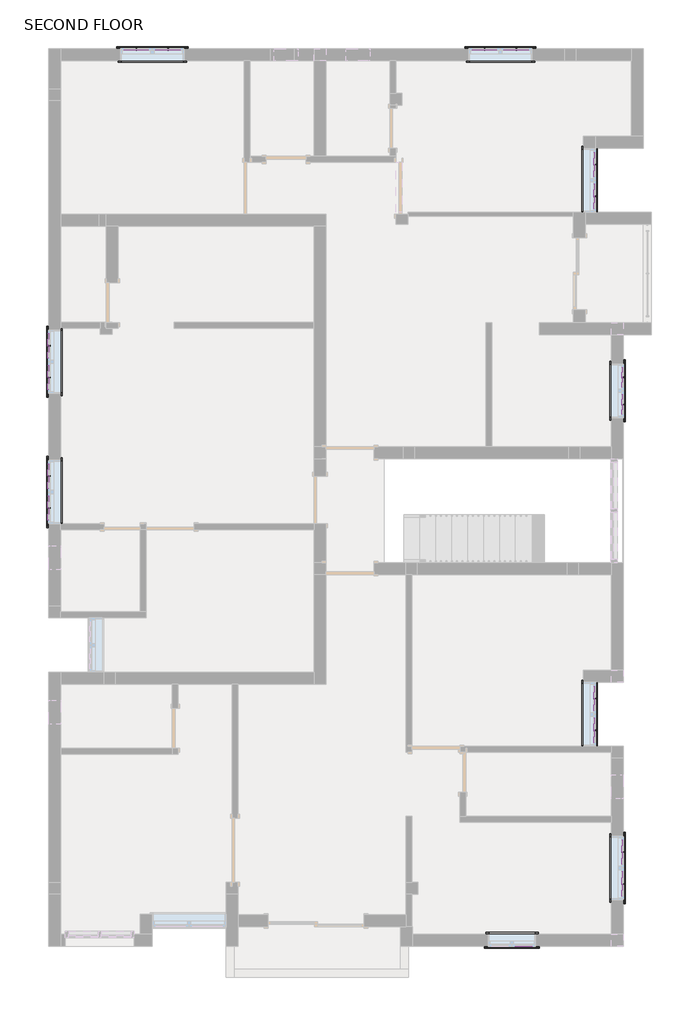
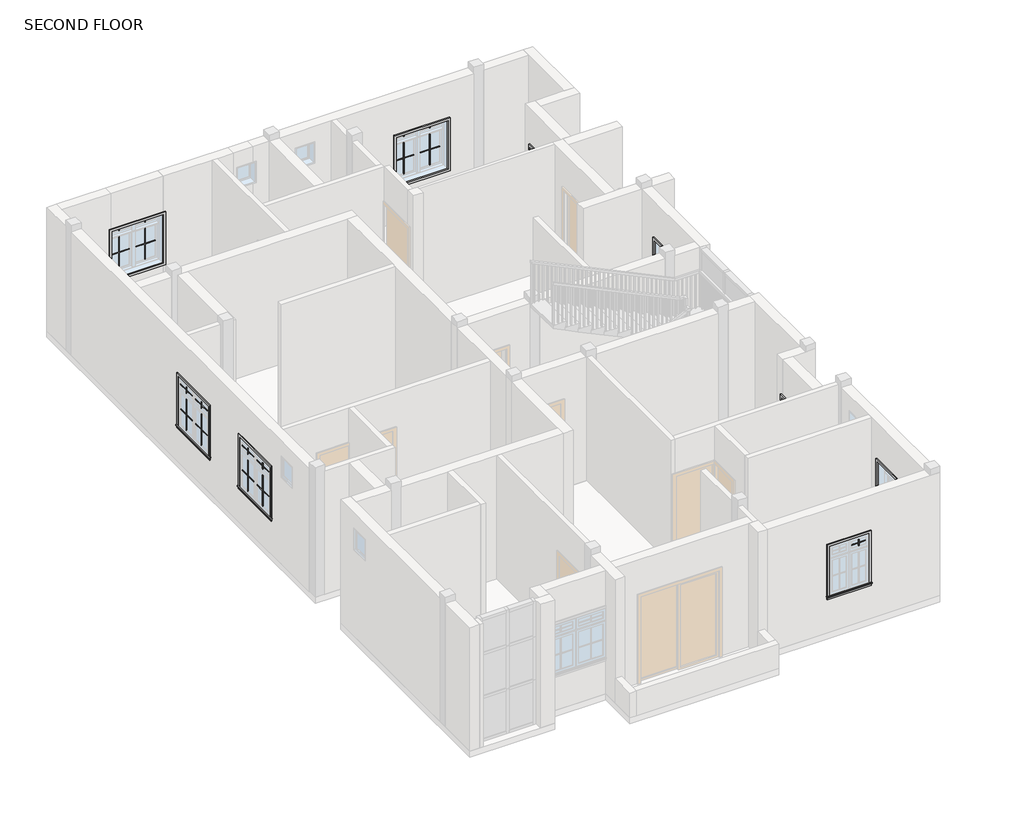
# One storey, part 6 of 6: 51 proxies.
"""IFC4 building model written with IfcOpenShell, lengths in millimetres."""

from ifc_helpers import new_model, si_unit, origin, place, context, project, spatial, transform, mapped, element, save
from components import muntin_pattern_2x2_muntin_pattern_2x2_2357e71d, muntin_pattern_2x2_muntin_pattern_2x2_302d8f29, muntin_pattern_2x2_muntin_pattern_2x2_3df65231, muntin_pattern_2x2_muntin_pattern_2x2_4af9dbf3, muntin_pattern_2x2_muntin_pattern_2x2_972acb6d, muntin_pattern_2x2_muntin_pattern_2x2_4879a4f3, muntin_pattern_2x2_muntin_pattern_2x2_604ffb00, trim_window_exterior_flat_with_sill_7cfdd449, trim_window_exterior_flat_with_sill_29d7a895, trim_window_exterior_flat_with_sill_e4b28ec3, trim_window_interior_flat_picture_frame_f1e0b15b, trim_window_interior_flat_picture_frame_56711e78, trim_window_interior_flat_picture_frame_39ff4276

model = new_model("IFC4")

# Units and contexts
model_context = context("Model", 3, world=origin())
ifc_project = project(units=[si_unit("LENGTHUNIT", "METRE", prefix="MILLI")], contexts=[model_context])

# Site, building, storey
site = spatial("IfcSite", under=ifc_project)
building = spatial("IfcBuilding", under=site)
storey = spatial("IfcBuildingStorey", under=building, Name="SECOND FLOOR", Elevation=6400.8)

# Proxies
placement = place(None, origin())
muntin_pattern_2x2_muntin_pattern_2x2_shape = muntin_pattern_2x2_muntin_pattern_2x2_2357e71d(model_context)
element("IfcBuildingElementProxy", 1, Name="Muntin Pattern_2x2 : Muntin Pattern_2x2", ObjectType="Muntin Pattern_2x2 : Muntin Pattern_2x2", at=placement, inside=storey, context=model_context, shape_type="MappedRepresentation", body=[
    mapped(muntin_pattern_2x2_muntin_pattern_2x2_shape, transform((-5090.4990981, 9290.6537587, 7385.05), x_axis=(1.0, 0.0, 0.0), y_axis=(0.0, 1.0, 0.0), z_axis=(0.0, 0.0, 1.0))),
])
element("IfcBuildingElementProxy", 2, Name="Muntin Pattern_2x2 : Muntin Pattern_2x2", ObjectType="Muntin Pattern_2x2 : Muntin Pattern_2x2", at=placement, inside=storey, context=model_context, shape_type="MappedRepresentation", body=[
    mapped(muntin_pattern_2x2_muntin_pattern_2x2_shape, transform((3661.3884019, 7088.7912587, 7385.05), x_axis=(0.0, -1.0, 0.0), y_axis=(1.0, 0.0, 0.0), z_axis=(0.0, 0.0, 1.0))),
])
element("IfcBuildingElementProxy", 3, Name="Muntin Pattern_2x2 : Muntin Pattern_2x2", ObjectType="Muntin Pattern_2x2 : Muntin Pattern_2x2", at=placement, inside=storey, context=model_context, shape_type="MappedRepresentation", body=[
    mapped(muntin_pattern_2x2_muntin_pattern_2x2_shape, transform((3661.3884019, -3096.6087413, 7385.05), x_axis=(0.0, -1.0, 0.0), y_axis=(1.0, 0.0, 0.0), z_axis=(0.0, 0.0, 1.0))),
])
element("IfcBuildingElementProxy", 4, Name="Muntin Pattern_2x2 : Muntin Pattern_2x2", ObjectType="Muntin Pattern_2x2 : Muntin Pattern_2x2", at=placement, inside=storey, context=model_context, shape_type="MappedRepresentation", body=[
    mapped(muntin_pattern_2x2_muntin_pattern_2x2_shape, transform((4194.7884019, -6025.7255734, 7385.05), x_axis=(0.0, -1.0, 0.0), y_axis=(1.0, 0.0, 0.0), z_axis=(0.0, 0.0, 1.0))),
])
element("IfcBuildingElementProxy", 5, Name="Muntin Pattern_2x2 : Muntin Pattern_2x2", ObjectType="Muntin Pattern_2x2 : Muntin Pattern_2x2", at=placement, inside=storey, context=model_context, shape_type="MappedRepresentation", body=[
    mapped(muntin_pattern_2x2_muntin_pattern_2x2_shape, transform((-6758.9615981, 538.7662587, 7385.05), x_axis=(0.0, 1.0, 0.0), y_axis=(-1.0, 0.0, 0.0), z_axis=(0.0, 0.0, 1.0))),
])
element("IfcBuildingElementProxy", 6, Name="Muntin Pattern_2x2 : Muntin Pattern_2x2", ObjectType="Muntin Pattern_2x2 : Muntin Pattern_2x2", at=placement, inside=storey, context=model_context, shape_type="MappedRepresentation", body=[
    mapped(muntin_pattern_2x2_muntin_pattern_2x2_shape, transform((-6758.9615981, 3024.5447861, 7385.05), x_axis=(0.0, 1.0, 0.0), y_axis=(-1.0, 0.0, 0.0), z_axis=(0.0, 0.0, 1.0))),
])
element("IfcBuildingElementProxy", 7, Name="Muntin Pattern_2x2 : Muntin Pattern_2x2", ObjectType="Muntin Pattern_2x2 : Muntin Pattern_2x2", at=placement, inside=storey, context=model_context, shape_type="MappedRepresentation", body=[
    mapped(muntin_pattern_2x2_muntin_pattern_2x2_shape, transform((1554.8452655, 9290.6537587, 7385.05), x_axis=(1.0, 0.0, 0.0), y_axis=(0.0, 1.0, 0.0), z_axis=(0.0, 0.0, 1.0))),
])
muntin_pattern_2x2_muntin_pattern_2x2_2_shape = muntin_pattern_2x2_muntin_pattern_2x2_302d8f29(model_context)
element("IfcBuildingElementProxy", 8, Name="Muntin Pattern_2x2 : Muntin Pattern_2x2", ObjectType="Muntin Pattern_2x2 : Muntin Pattern_2x2", at=placement, inside=storey, context=model_context, shape_type="MappedRepresentation", body=[
    mapped(muntin_pattern_2x2_muntin_pattern_2x2_2_shape, transform((-4484.0740981, 9290.6537587, 7385.05), x_axis=(-1.0, 0.0, 0.0), y_axis=(0.0, -1.0, 0.0), z_axis=(0.0, 0.0, 1.0))),
])
element("IfcBuildingElementProxy", 9, Name="Muntin Pattern_2x2 : Muntin Pattern_2x2", ObjectType="Muntin Pattern_2x2 : Muntin Pattern_2x2", at=placement, inside=storey, context=model_context, shape_type="MappedRepresentation", body=[
    mapped(muntin_pattern_2x2_muntin_pattern_2x2_2_shape, transform((3661.3884019, 6482.3662587, 7385.05), x_axis=(0.0, 1.0, 0.0), y_axis=(-1.0, 0.0, 0.0), z_axis=(0.0, 0.0, 1.0))),
])
element("IfcBuildingElementProxy", 10, Name="Muntin Pattern_2x2 : Muntin Pattern_2x2", ObjectType="Muntin Pattern_2x2 : Muntin Pattern_2x2", at=placement, inside=storey, context=model_context, shape_type="MappedRepresentation", body=[
    mapped(muntin_pattern_2x2_muntin_pattern_2x2_2_shape, transform((3661.3884019, -3703.0337413, 7385.05), x_axis=(0.0, 1.0, 0.0), y_axis=(-1.0, 0.0, 0.0), z_axis=(0.0, 0.0, 1.0))),
])
element("IfcBuildingElementProxy", 11, Name="Muntin Pattern_2x2 : Muntin Pattern_2x2", ObjectType="Muntin Pattern_2x2 : Muntin Pattern_2x2", at=placement, inside=storey, context=model_context, shape_type="MappedRepresentation", body=[
    mapped(muntin_pattern_2x2_muntin_pattern_2x2_2_shape, transform((4194.7884019, -6632.1505734, 7385.05), x_axis=(0.0, 1.0, 0.0), y_axis=(-1.0, 0.0, 0.0), z_axis=(0.0, 0.0, 1.0))),
])
element("IfcBuildingElementProxy", 12, Name="Muntin Pattern_2x2 : Muntin Pattern_2x2", ObjectType="Muntin Pattern_2x2 : Muntin Pattern_2x2", at=placement, inside=storey, context=model_context, shape_type="MappedRepresentation", body=[
    mapped(muntin_pattern_2x2_muntin_pattern_2x2_2_shape, transform((-6758.9615981, 1145.1912587, 7385.05), x_axis=(0.0, -1.0, 0.0), y_axis=(1.0, 0.0, 0.0), z_axis=(0.0, 0.0, 1.0))),
])
element("IfcBuildingElementProxy", 13, Name="Muntin Pattern_2x2 : Muntin Pattern_2x2", ObjectType="Muntin Pattern_2x2 : Muntin Pattern_2x2", at=placement, inside=storey, context=model_context, shape_type="MappedRepresentation", body=[
    mapped(muntin_pattern_2x2_muntin_pattern_2x2_2_shape, transform((-6758.9615981, 3630.9697861, 7385.05), x_axis=(0.0, -1.0, 0.0), y_axis=(1.0, 0.0, 0.0), z_axis=(0.0, 0.0, 1.0))),
])
element("IfcBuildingElementProxy", 14, Name="Muntin Pattern_2x2 : Muntin Pattern_2x2", ObjectType="Muntin Pattern_2x2 : Muntin Pattern_2x2", at=placement, inside=storey, context=model_context, shape_type="MappedRepresentation", body=[
    mapped(muntin_pattern_2x2_muntin_pattern_2x2_2_shape, transform((2161.2702655, 9290.6537587, 7385.05), x_axis=(-1.0, 0.0, 0.0), y_axis=(0.0, -1.0, 0.0), z_axis=(0.0, 0.0, 1.0))),
])
muntin_pattern_2x2_muntin_pattern_2x2_3_shape = muntin_pattern_2x2_muntin_pattern_2x2_3df65231(model_context)
element("IfcBuildingElementProxy", 15, Name="Muntin Pattern_2x2 : Muntin Pattern_2x2", ObjectType="Muntin Pattern_2x2 : Muntin Pattern_2x2", at=placement, inside=storey, context=model_context, shape_type="MappedRepresentation", body=[
    mapped(muntin_pattern_2x2_muntin_pattern_2x2_3_shape, transform((-4484.0740981, 9290.6537587, 8299.45), x_axis=(-1.0, 0.0, 0.0), y_axis=(0.0, -1.0, 0.0), z_axis=(0.0, 0.0, 1.0))),
])
element("IfcBuildingElementProxy", 16, Name="Muntin Pattern_2x2 : Muntin Pattern_2x2", ObjectType="Muntin Pattern_2x2 : Muntin Pattern_2x2", at=placement, inside=storey, context=model_context, shape_type="MappedRepresentation", body=[
    mapped(muntin_pattern_2x2_muntin_pattern_2x2_3_shape, transform((-5090.4990981, 9290.6537587, 8299.45), x_axis=(-1.0, 0.0, 0.0), y_axis=(0.0, -1.0, 0.0), z_axis=(0.0, 0.0, 1.0))),
])
element("IfcBuildingElementProxy", 17, Name="Muntin Pattern_2x2 : Muntin Pattern_2x2", ObjectType="Muntin Pattern_2x2 : Muntin Pattern_2x2", at=placement, inside=storey, context=model_context, shape_type="MappedRepresentation", body=[
    mapped(muntin_pattern_2x2_muntin_pattern_2x2_3_shape, transform((3661.3884019, 6482.3662587, 8299.45), x_axis=(0.0, 1.0, 0.0), y_axis=(-1.0, 0.0, 0.0), z_axis=(0.0, 0.0, 1.0))),
])
element("IfcBuildingElementProxy", 18, Name="Muntin Pattern_2x2 : Muntin Pattern_2x2", ObjectType="Muntin Pattern_2x2 : Muntin Pattern_2x2", at=placement, inside=storey, context=model_context, shape_type="MappedRepresentation", body=[
    mapped(muntin_pattern_2x2_muntin_pattern_2x2_3_shape, transform((3661.3884019, 7088.7912587, 8299.45), x_axis=(0.0, 1.0, 0.0), y_axis=(-1.0, 0.0, 0.0), z_axis=(0.0, 0.0, 1.0))),
])
element("IfcBuildingElementProxy", 19, Name="Muntin Pattern_2x2 : Muntin Pattern_2x2", ObjectType="Muntin Pattern_2x2 : Muntin Pattern_2x2", at=placement, inside=storey, context=model_context, shape_type="MappedRepresentation", body=[
    mapped(muntin_pattern_2x2_muntin_pattern_2x2_3_shape, transform((3661.3884019, -3703.0337413, 8299.45), x_axis=(0.0, 1.0, 0.0), y_axis=(-1.0, 0.0, 0.0), z_axis=(0.0, 0.0, 1.0))),
])
element("IfcBuildingElementProxy", 20, Name="Muntin Pattern_2x2 : Muntin Pattern_2x2", ObjectType="Muntin Pattern_2x2 : Muntin Pattern_2x2", at=placement, inside=storey, context=model_context, shape_type="MappedRepresentation", body=[
    mapped(muntin_pattern_2x2_muntin_pattern_2x2_3_shape, transform((3661.3884019, -3096.6087413, 8299.45), x_axis=(0.0, 1.0, 0.0), y_axis=(-1.0, 0.0, 0.0), z_axis=(0.0, 0.0, 1.0))),
])
element("IfcBuildingElementProxy", 21, Name="Muntin Pattern_2x2 : Muntin Pattern_2x2", ObjectType="Muntin Pattern_2x2 : Muntin Pattern_2x2", at=placement, inside=storey, context=model_context, shape_type="MappedRepresentation", body=[
    mapped(muntin_pattern_2x2_muntin_pattern_2x2_3_shape, transform((4194.7884019, -6632.1505734, 8299.45), x_axis=(0.0, 1.0, 0.0), y_axis=(-1.0, 0.0, 0.0), z_axis=(0.0, 0.0, 1.0))),
])
element("IfcBuildingElementProxy", 22, Name="Muntin Pattern_2x2 : Muntin Pattern_2x2", ObjectType="Muntin Pattern_2x2 : Muntin Pattern_2x2", at=placement, inside=storey, context=model_context, shape_type="MappedRepresentation", body=[
    mapped(muntin_pattern_2x2_muntin_pattern_2x2_3_shape, transform((4194.7884019, -6025.7255734, 8299.45), x_axis=(0.0, 1.0, 0.0), y_axis=(-1.0, 0.0, 0.0), z_axis=(0.0, 0.0, 1.0))),
])
element("IfcBuildingElementProxy", 23, Name="Muntin Pattern_2x2 : Muntin Pattern_2x2", ObjectType="Muntin Pattern_2x2 : Muntin Pattern_2x2", at=placement, inside=storey, context=model_context, shape_type="MappedRepresentation", body=[
    mapped(muntin_pattern_2x2_muntin_pattern_2x2_3_shape, transform((-6758.9615981, 1145.1912587, 8299.45), x_axis=(0.0, -1.0, 0.0), y_axis=(1.0, 0.0, 0.0), z_axis=(0.0, 0.0, 1.0))),
])
element("IfcBuildingElementProxy", 24, Name="Muntin Pattern_2x2 : Muntin Pattern_2x2", ObjectType="Muntin Pattern_2x2 : Muntin Pattern_2x2", at=placement, inside=storey, context=model_context, shape_type="MappedRepresentation", body=[
    mapped(muntin_pattern_2x2_muntin_pattern_2x2_3_shape, transform((-6758.9615981, 538.7662587, 8299.45), x_axis=(0.0, -1.0, 0.0), y_axis=(1.0, 0.0, 0.0), z_axis=(0.0, 0.0, 1.0))),
])
element("IfcBuildingElementProxy", 25, Name="Muntin Pattern_2x2 : Muntin Pattern_2x2", ObjectType="Muntin Pattern_2x2 : Muntin Pattern_2x2", at=placement, inside=storey, context=model_context, shape_type="MappedRepresentation", body=[
    mapped(muntin_pattern_2x2_muntin_pattern_2x2_3_shape, transform((-6758.9615981, 3630.9697861, 8299.45), x_axis=(0.0, -1.0, 0.0), y_axis=(1.0, 0.0, 0.0), z_axis=(0.0, 0.0, 1.0))),
])
element("IfcBuildingElementProxy", 26, Name="Muntin Pattern_2x2 : Muntin Pattern_2x2", ObjectType="Muntin Pattern_2x2 : Muntin Pattern_2x2", at=placement, inside=storey, context=model_context, shape_type="MappedRepresentation", body=[
    mapped(muntin_pattern_2x2_muntin_pattern_2x2_3_shape, transform((-6758.9615981, 3024.5447861, 8299.45), x_axis=(0.0, -1.0, 0.0), y_axis=(1.0, 0.0, 0.0), z_axis=(0.0, 0.0, 1.0))),
])
element("IfcBuildingElementProxy", 27, Name="Muntin Pattern_2x2 : Muntin Pattern_2x2", ObjectType="Muntin Pattern_2x2 : Muntin Pattern_2x2", at=placement, inside=storey, context=model_context, shape_type="MappedRepresentation", body=[
    mapped(muntin_pattern_2x2_muntin_pattern_2x2_3_shape, transform((2161.2702655, 9290.6537587, 8299.45), x_axis=(-1.0, 0.0, 0.0), y_axis=(0.0, -1.0, 0.0), z_axis=(0.0, 0.0, 1.0))),
])
element("IfcBuildingElementProxy", 28, Name="Muntin Pattern_2x2 : Muntin Pattern_2x2", ObjectType="Muntin Pattern_2x2 : Muntin Pattern_2x2", at=placement, inside=storey, context=model_context, shape_type="MappedRepresentation", body=[
    mapped(muntin_pattern_2x2_muntin_pattern_2x2_3_shape, transform((1554.8452655, 9290.6537587, 8299.45), x_axis=(-1.0, 0.0, 0.0), y_axis=(0.0, -1.0, 0.0), z_axis=(0.0, 0.0, 1.0))),
])
muntin_pattern_2x2_muntin_pattern_2x2_4_shape = muntin_pattern_2x2_muntin_pattern_2x2_4af9dbf3(model_context)
element("IfcBuildingElementProxy", 29, Name="Muntin Pattern_2x2 : Muntin Pattern_2x2", ObjectType="Muntin Pattern_2x2 : Muntin Pattern_2x2", at=placement, inside=storey, context=model_context, shape_type="MappedRepresentation", body=[
    mapped(muntin_pattern_2x2_muntin_pattern_2x2_4_shape, transform((4194.7884019, 3031.1412587, 7385.05), x_axis=(0.0, -1.0, 0.0), y_axis=(1.0, 0.0, 0.0), z_axis=(0.0, 0.0, 1.0))),
])
muntin_pattern_2x2_muntin_pattern_2x2_5_shape = muntin_pattern_2x2_muntin_pattern_2x2_972acb6d(model_context)
element("IfcBuildingElementProxy", 30, Name="Muntin Pattern_2x2 : Muntin Pattern_2x2", ObjectType="Muntin Pattern_2x2 : Muntin Pattern_2x2", at=placement, inside=storey, context=model_context, shape_type="MappedRepresentation", body=[
    mapped(muntin_pattern_2x2_muntin_pattern_2x2_5_shape, transform((4194.7884019, 2513.6162587, 7385.05), x_axis=(0.0, 1.0, 0.0), y_axis=(-1.0, 0.0, 0.0), z_axis=(0.0, 0.0, 1.0))),
])
muntin_pattern_2x2_muntin_pattern_2x2_6_shape = muntin_pattern_2x2_muntin_pattern_2x2_4879a4f3(model_context)
element("IfcBuildingElementProxy", 31, Name="Muntin Pattern_2x2 : Muntin Pattern_2x2", ObjectType="Muntin Pattern_2x2 : Muntin Pattern_2x2", at=placement, inside=storey, context=model_context, shape_type="MappedRepresentation", body=[
    mapped(muntin_pattern_2x2_muntin_pattern_2x2_6_shape, transform((4194.7884019, 2513.6162587, 8299.45), x_axis=(0.0, 1.0, 0.0), y_axis=(-1.0, 0.0, 0.0), z_axis=(0.0, 0.0, 1.0))),
])
element("IfcBuildingElementProxy", 32, Name="Muntin Pattern_2x2 : Muntin Pattern_2x2", ObjectType="Muntin Pattern_2x2 : Muntin Pattern_2x2", at=placement, inside=storey, context=model_context, shape_type="MappedRepresentation", body=[
    mapped(muntin_pattern_2x2_muntin_pattern_2x2_6_shape, transform((4194.7884019, 3031.1412587, 8299.45), x_axis=(0.0, 1.0, 0.0), y_axis=(-1.0, 0.0, 0.0), z_axis=(0.0, 0.0, 1.0))),
])
muntin_pattern_2x2_muntin_pattern_2x2_7_shape = muntin_pattern_2x2_muntin_pattern_2x2_604ffb00(model_context)
element("IfcBuildingElementProxy", 33, Name="Muntin Pattern_2x2 : Muntin Pattern_2x2", ObjectType="Muntin Pattern_2x2 : Muntin Pattern_2x2", at=placement, inside=storey, context=model_context, shape_type="MappedRepresentation", body=[
    mapped(muntin_pattern_2x2_muntin_pattern_2x2_7_shape, transform((2304.0759019, -7809.8962413, 8299.45), x_axis=(1.0, 0.0, 0.0), y_axis=(0.0, 1.0, 0.0), z_axis=(0.0, 0.0, 1.0))),
])
trim_window_exterior_flat_with_sill_shape = trim_window_exterior_flat_with_sill_7cfdd449(model_context)
element("IfcBuildingElementProxy", 34, Name="Trim-Window-Exterior-Flat : with Sill", ObjectType="Trim-Window-Exterior-Flat : with Sill", at=placement, inside=storey, context=model_context, shape_type="MappedRepresentation", body=[
    mapped(trim_window_exterior_flat_with_sill_shape, transform((-4787.2865981, 9300.1787587, 8534.4), x_axis=(-1.0, 0.0, 0.0), y_axis=(0.0, 0.0, 1.0), z_axis=(0.0, 1.0, 0.0))),
])
element("IfcBuildingElementProxy", 35, Name="Trim-Window-Exterior-Flat : with Sill", ObjectType="Trim-Window-Exterior-Flat : with Sill", at=placement, inside=storey, context=model_context, shape_type="MappedRepresentation", body=[
    mapped(trim_window_exterior_flat_with_sill_shape, transform((3670.9134019, 6785.5787587, 8534.4), x_axis=(0.0, 1.0, 0.0), y_axis=(0.0, 0.0, 1.0), z_axis=(1.0, 0.0, 0.0))),
])
element("IfcBuildingElementProxy", 36, Name="Trim-Window-Exterior-Flat : with Sill", ObjectType="Trim-Window-Exterior-Flat : with Sill", at=placement, inside=storey, context=model_context, shape_type="MappedRepresentation", body=[
    mapped(trim_window_exterior_flat_with_sill_shape, transform((3670.9134019, -3399.8212413, 8534.4), x_axis=(0.0, 1.0, 0.0), y_axis=(0.0, 0.0, 1.0), z_axis=(1.0, 0.0, 0.0))),
])
element("IfcBuildingElementProxy", 37, Name="Trim-Window-Exterior-Flat : with Sill", ObjectType="Trim-Window-Exterior-Flat : with Sill", at=placement, inside=storey, context=model_context, shape_type="MappedRepresentation", body=[
    mapped(trim_window_exterior_flat_with_sill_shape, transform((4204.3134019, -6328.9380734, 8534.4), x_axis=(0.0, 1.0, 0.0), y_axis=(0.0, 0.0, 1.0), z_axis=(1.0, 0.0, 0.0))),
])
element("IfcBuildingElementProxy", 38, Name="Trim-Window-Exterior-Flat : with Sill", ObjectType="Trim-Window-Exterior-Flat : with Sill", at=placement, inside=storey, context=model_context, shape_type="MappedRepresentation", body=[
    mapped(trim_window_exterior_flat_with_sill_shape, transform((-6768.4865981, 841.9787587, 8534.4), x_axis=(0.0, -1.0, 0.0), y_axis=(0.0, 0.0, 1.0), z_axis=(-1.0, 0.0, 0.0))),
])
element("IfcBuildingElementProxy", 39, Name="Trim-Window-Exterior-Flat : with Sill", ObjectType="Trim-Window-Exterior-Flat : with Sill", at=placement, inside=storey, context=model_context, shape_type="MappedRepresentation", body=[
    mapped(trim_window_exterior_flat_with_sill_shape, transform((-6768.4865981, 3327.7572861, 8534.4), x_axis=(0.0, -1.0, 0.0), y_axis=(0.0, 0.0, 1.0), z_axis=(-1.0, 0.0, 0.0))),
])
element("IfcBuildingElementProxy", 40, Name="Trim-Window-Exterior-Flat : with Sill", ObjectType="Trim-Window-Exterior-Flat : with Sill", at=placement, inside=storey, context=model_context, shape_type="MappedRepresentation", body=[
    mapped(trim_window_exterior_flat_with_sill_shape, transform((1858.0577655, 9300.1787587, 8534.4), x_axis=(-1.0, 0.0, 0.0), y_axis=(0.0, 0.0, 1.0), z_axis=(0.0, 1.0, 0.0))),
])
trim_window_exterior_flat_with_sill_2_shape = trim_window_exterior_flat_with_sill_29d7a895(model_context)
element("IfcBuildingElementProxy", 41, Name="Trim-Window-Exterior-Flat : with Sill", ObjectType="Trim-Window-Exterior-Flat : with Sill", at=placement, inside=storey, context=model_context, shape_type="MappedRepresentation", body=[
    mapped(trim_window_exterior_flat_with_sill_2_shape, transform((4204.3134019, 2772.3787587, 8534.4), x_axis=(0.0, 1.0, 0.0), y_axis=(0.0, 0.0, 1.0), z_axis=(1.0, 0.0, 0.0))),
])
trim_window_exterior_flat_with_sill_3_shape = trim_window_exterior_flat_with_sill_e4b28ec3(model_context)
element("IfcBuildingElementProxy", 42, Name="Trim-Window-Exterior-Flat : with Sill", ObjectType="Trim-Window-Exterior-Flat : with Sill", at=placement, inside=storey, context=model_context, shape_type="MappedRepresentation", body=[
    mapped(trim_window_exterior_flat_with_sill_3_shape, transform((2077.0634019, -7819.4212413, 8534.4), x_axis=(1.0, 0.0, 0.0), y_axis=(0.0, 0.0, 1.0), z_axis=(0.0, -1.0, 0.0))),
])
trim_window_interior_flat_picture_frame_shape = trim_window_interior_flat_picture_frame_f1e0b15b(model_context)
element("IfcBuildingElementProxy", 43, Name="Trim-Window-Interior-Flat : Picture Frame", ObjectType="Trim-Window-Interior-Flat : Picture Frame", at=placement, inside=storey, context=model_context, shape_type="MappedRepresentation", body=[
    mapped(trim_window_interior_flat_picture_frame_shape, transform((-4787.2865981, 9071.5787587, 8534.4), x_axis=(1.0, 0.0, 0.0), y_axis=(0.0, 0.0, 1.0), z_axis=(0.0, -1.0, 0.0))),
])
element("IfcBuildingElementProxy", 44, Name="Trim-Window-Interior-Flat : Picture Frame", ObjectType="Trim-Window-Interior-Flat : Picture Frame", at=placement, inside=storey, context=model_context, shape_type="MappedRepresentation", body=[
    mapped(trim_window_interior_flat_picture_frame_shape, transform((3442.3134019, 6785.5787587, 8534.4), x_axis=(0.0, -1.0, 0.0), y_axis=(0.0, 0.0, 1.0), z_axis=(-1.0, 0.0, 0.0))),
])
element("IfcBuildingElementProxy", 45, Name="Trim-Window-Interior-Flat : Picture Frame", ObjectType="Trim-Window-Interior-Flat : Picture Frame", at=placement, inside=storey, context=model_context, shape_type="MappedRepresentation", body=[
    mapped(trim_window_interior_flat_picture_frame_shape, transform((3442.3134019, -3399.8212413, 8534.4), x_axis=(0.0, -1.0, 0.0), y_axis=(0.0, 0.0, 1.0), z_axis=(-1.0, 0.0, 0.0))),
])
element("IfcBuildingElementProxy", 46, Name="Trim-Window-Interior-Flat : Picture Frame", ObjectType="Trim-Window-Interior-Flat : Picture Frame", at=placement, inside=storey, context=model_context, shape_type="MappedRepresentation", body=[
    mapped(trim_window_interior_flat_picture_frame_shape, transform((3975.7134019, -6328.9380734, 8534.4), x_axis=(0.0, -1.0, 0.0), y_axis=(0.0, 0.0, 1.0), z_axis=(-1.0, 0.0, 0.0))),
])
element("IfcBuildingElementProxy", 47, Name="Trim-Window-Interior-Flat : Picture Frame", ObjectType="Trim-Window-Interior-Flat : Picture Frame", at=placement, inside=storey, context=model_context, shape_type="MappedRepresentation", body=[
    mapped(trim_window_interior_flat_picture_frame_shape, transform((-6539.8865981, 841.9787587, 8534.4), x_axis=(0.0, 1.0, 0.0), y_axis=(0.0, 0.0, 1.0), z_axis=(1.0, 0.0, 0.0))),
])
element("IfcBuildingElementProxy", 48, Name="Trim-Window-Interior-Flat : Picture Frame", ObjectType="Trim-Window-Interior-Flat : Picture Frame", at=placement, inside=storey, context=model_context, shape_type="MappedRepresentation", body=[
    mapped(trim_window_interior_flat_picture_frame_shape, transform((-6539.8865981, 3327.7572861, 8534.4), x_axis=(0.0, 1.0, 0.0), y_axis=(0.0, 0.0, 1.0), z_axis=(1.0, 0.0, 0.0))),
])
element("IfcBuildingElementProxy", 49, Name="Trim-Window-Interior-Flat : Picture Frame", ObjectType="Trim-Window-Interior-Flat : Picture Frame", at=placement, inside=storey, context=model_context, shape_type="MappedRepresentation", body=[
    mapped(trim_window_interior_flat_picture_frame_shape, transform((1858.0577655, 9071.5787587, 8534.4), x_axis=(1.0, 0.0, 0.0), y_axis=(0.0, 0.0, 1.0), z_axis=(0.0, -1.0, 0.0))),
])
trim_window_interior_flat_picture_frame_2_shape = trim_window_interior_flat_picture_frame_56711e78(model_context)
element("IfcBuildingElementProxy", 50, Name="Trim-Window-Interior-Flat : Picture Frame", ObjectType="Trim-Window-Interior-Flat : Picture Frame", at=placement, inside=storey, context=model_context, shape_type="MappedRepresentation", body=[
    mapped(trim_window_interior_flat_picture_frame_2_shape, transform((3975.7134019, 2772.3787587, 8534.4), x_axis=(0.0, -1.0, 0.0), y_axis=(0.0, 0.0, 1.0), z_axis=(-1.0, 0.0, 0.0))),
])
trim_window_interior_flat_picture_frame_3_shape = trim_window_interior_flat_picture_frame_39ff4276(model_context)
element("IfcBuildingElementProxy", 51, Name="Trim-Window-Interior-Flat : Picture Frame", ObjectType="Trim-Window-Interior-Flat : Picture Frame", at=placement, inside=storey, context=model_context, shape_type="MappedRepresentation", body=[
    mapped(trim_window_interior_flat_picture_frame_3_shape, transform((2077.0634019, -7590.8212413, 8534.4), x_axis=(-1.0, 0.0, 0.0), y_axis=(0.0, 0.0, 1.0), z_axis=(0.0, 1.0, 0.0))),
])

save(model, "model.ifc")

# Revit data of these elements
# Type "Muntin Pattern_2x2 : Muntin Pattern_2x2"
#   Width [instance default] = 4' - 0"
#   Thickness = 0' - 0 1/2"
#   Height [instance default] = 4' - 0"
#   Distance = 0' - 0 3/4"
#   Interior Material [instance default] = none
#   Exterior Material [instance default] = none
#   Default Elevation = 0
# Type "Trim-Window-Exterior-Flat : with Sill"
#   Trim Width = 0' - 2 1/4"
#   Trim Thickness_Picture Frame = 0' - 1 1/4"
#   Trim Thickness_with Sill = 0' - 0 3/4"
#   Sill Thickness = 0' - 1 1/4"
#   Opening Width [instance default] = 2' - 0"
#   Opening Height [instance default] = 3' - 0"
#   Default Elevation = 4' - 0"
#   Sill = yes
#   Picture Frame = no
#   Trim Material [instance default] = none
# Type "Trim-Window-Interior-Flat : Picture Frame"
#   Trim Thickness_Picture Frame = 0' - 1 1/4"
#   Trim Width = 0' - 2 1/4"
#   Trim Thickness_with Sill = 0' - 0 3/4"
#   Sill Thickness = 0' - 1 1/4"
#   Opening Width [instance default] = 2' - 0"
#   Opening Height [instance default] = 3' - 0"
#   Default Elevation = 4' - 0"
#   Sill = no
#   Picture Frame = yes
#   Trim Material [instance default] = none
# Elements 1, 2, 3, 4, 5, 6, 7, 8, 9, 10, 11, 12, 13, 14 (IfcBuildingElementProxy, "Muntin Pattern_2x2 : Muntin Pattern_2x2")
#   Width = 1' - 6 5/8"
#   Height = 2' - 6 1/2"
#   Interior Material = Wood - Stained
#   Exterior Material = Clad - White
#   Phase Created = New Construction
#   Materials on its faces: "Clad - White", "Wood - Stained"
# Elements 15, 16, 17, 18, 19, 20, 21, 22, 23, 24, 25, 26, 27, 28 (IfcBuildingElementProxy, "Muntin Pattern_2x2 : Muntin Pattern_2x2")
#   Width = 1' - 6 5/8"
#   Height = 0' - 6 1/2"
#   Interior Material = Wood - Stained
#   Exterior Material = Clad - White
#   Phase Created = New Construction
#   Materials on its faces: "Clad - White", "Wood - Stained"
# Elements 29, 30 (IfcBuildingElementProxy, "Muntin Pattern_2x2 : Muntin Pattern_2x2")
#   Width = 1' - 3 1/8"
#   Height = 2' - 6 1/2"
#   Interior Material = Wood - Stained
#   Exterior Material = Clad - White
#   Phase Created = New Construction
#   Materials on its faces: "Clad - White", "Wood - Stained"
# Elements 31, 32 (IfcBuildingElementProxy, "Muntin Pattern_2x2 : Muntin Pattern_2x2")
#   Width = 1' - 3 1/8"
#   Height = 0' - 6 1/2"
#   Interior Material = Wood - Stained
#   Exterior Material = Clad - White
#   Phase Created = New Construction
#   Materials on its faces: "Clad - White", "Wood - Stained"
# Element 33 (IfcBuildingElementProxy, "Muntin Pattern_2x2 : Muntin Pattern_2x2")
#   Width = 1' - 0 5/8"
#   Height = 0' - 6 1/2"
#   Interior Material = Wood - Stained
#   Exterior Material = Clad - White
#   Phase Created = New Construction
#   Materials on its faces: "Clad - White", "Wood - Stained"
# Elements 34, 35, 36, 37, 38, 39, 40 (IfcBuildingElementProxy, "Trim-Window-Exterior-Flat : with Sill")
#   Opening Width = 4' - 0"
#   Opening Height = 4' - 0"
#   Trim Material = Clad - White
#   Phase Created = New Construction
#   Materials on its faces: "Clad - White"
# Element 41 (IfcBuildingElementProxy, "Trim-Window-Exterior-Flat : with Sill")
#   Opening Width = 3' - 5"
#   Opening Height = 4' - 0"
#   Trim Material = Clad - White
#   Phase Created = New Construction
#   Materials on its faces: "Clad - White"
# Element 42 (IfcBuildingElementProxy, "Trim-Window-Exterior-Flat : with Sill")
#   Opening Width = 3' - 0"
#   Opening Height = 4' - 0"
#   Trim Material = Clad - White
#   Phase Created = New Construction
#   Materials on its faces: "Clad - White"
# Elements 43, 44, 45, 46, 47, 48, 49 (IfcBuildingElementProxy, "Trim-Window-Interior-Flat : Picture Frame")
#   Opening Width = 4' - 0"
#   Opening Height = 4' - 0"
#   Trim Material = Wood - Stained
#   Phase Created = New Construction
#   Materials on its faces: "Wood - Stained"
# Element 50 (IfcBuildingElementProxy, "Trim-Window-Interior-Flat : Picture Frame")
#   Opening Width = 3' - 5"
#   Opening Height = 4' - 0"
#   Trim Material = Wood - Stained
#   Phase Created = New Construction
#   Materials on its faces: "Wood - Stained"
# Element 51 (IfcBuildingElementProxy, "Trim-Window-Interior-Flat : Picture Frame")
#   Opening Width = 3' - 0"
#   Opening Height = 4' - 0"
#   Trim Material = Wood - Stained
#   Phase Created = New Construction
#   Materials on its faces: "Wood - Stained"
# Materials
#   "Clad - White": class "Wood", colour RGB 242 242 238, transparency 0, Cost = 0
#   "Wood - Stained": class "Wood", colour RGB 224 178 126, transparency 0, Cost = 0
